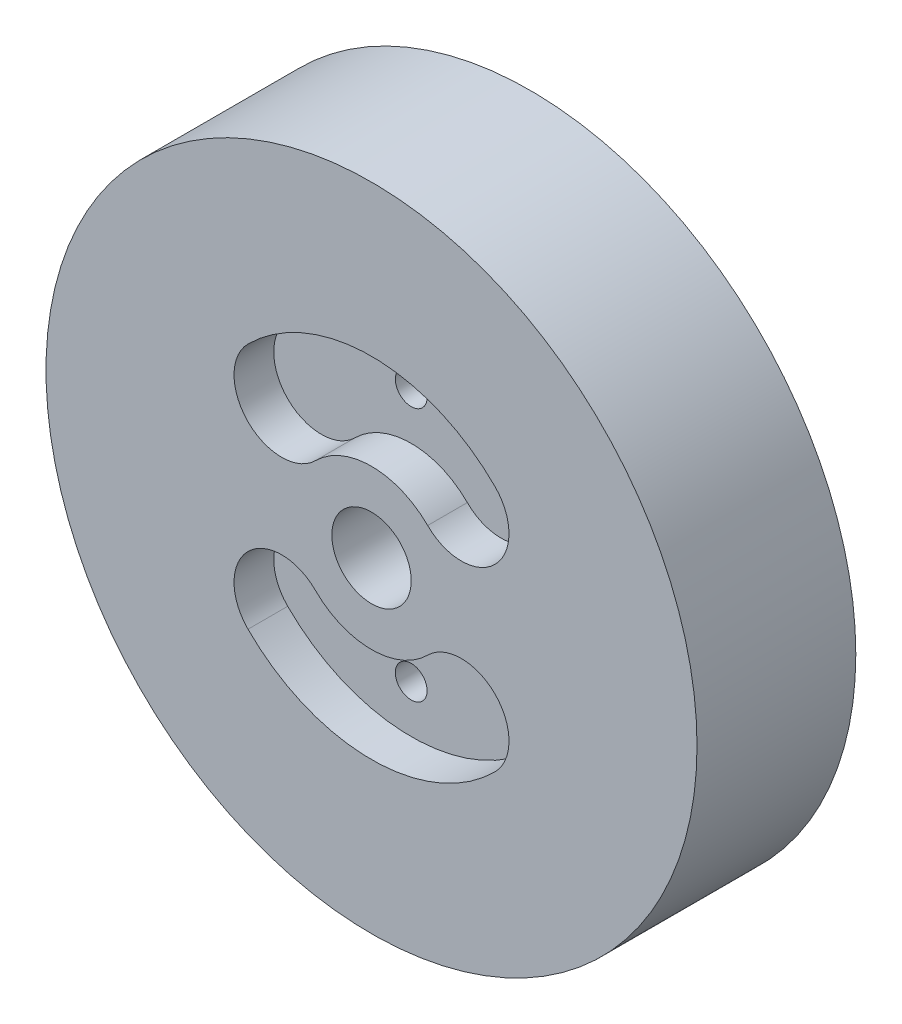
from build123d import *

# Parameters (mm, degrees)
DISC_PROFILE_41_R         = 20.5
PORT_BLOCK_DISC_DEPTH     = 10
ARC_PORT_SLOTS_DEPTH      = 2.5
THROUGH_PORTS_PROFILE_R   = 2.5
THROUGH_PORTS_PROFILE_R_2 = 1
THROUGH_PORTS_DEPTH       = 32.5
PORT_POCKETS_PROFILE_R    = 2.5
PORT_POCKETS_DEPTH        = 5


with BuildPart() as part:
    # Disc Profile Ø41 → Port Block Disc (new body)
    with BuildSketch(Plane.XY):
        Circle(DISC_PROFILE_41_R)
    extrude(amount=PORT_BLOCK_DISC_DEPTH)

    # Arc Port Slots Profile → Arc Port Slots (cut)
    with BuildSketch(Plane.XY.offset(10)):
        with BuildLine():
            ThreePointArc((7.778174593, 7.778174593), (0, 11), (-7.778174593, 7.778174593))
            ThreePointArc((-7.778174593, 7.778174593), (-7.778174593, 3.535533906), (-3.535533906, 3.535533906))
            ThreePointArc((-3.535533906, 3.535533906), (0, 5), (3.535533906, 3.535533906))
            ThreePointArc((3.535533906, 3.535533906), (7.778174593, 3.535533906), (7.778174593, 7.778174593))
        make_face()
        with BuildLine():
            ThreePointArc((3.535533906, -3.535533906), (0, -5), (-3.535533906, -3.535533906))
            ThreePointArc((-3.535533906, -3.535533906), (-7.778174593, -3.535533906), (-7.778174593, -7.778174593))
            ThreePointArc((-7.778174593, -7.778174593), (0, -11), (7.778174593, -7.778174593))
            ThreePointArc((7.778174593, -7.778174593), (7.778174593, -3.535533906), (3.535533906, -3.535533906))
        make_face()
    extrude(amount=-ARC_PORT_SLOTS_DEPTH, mode=Mode.SUBTRACT)

    # Through Ports Profile → Through Ports (cut)
    with BuildSketch(Plane.XY.offset(10)):
        Circle(THROUGH_PORTS_PROFILE_R)
        with Locations((0, 8)):
            Circle(THROUGH_PORTS_PROFILE_R_2)
        with Locations((0, -8)):
            Circle(THROUGH_PORTS_PROFILE_R_2)
    extrude(amount=-THROUGH_PORTS_DEPTH, mode=Mode.SUBTRACT)

    # Port Pockets Profile → Port Pockets (cut)
    with BuildSketch(Plane(origin=(0, 0, 0), x_dir=(-1, 0, 0), z_dir=(0, 0, -1))):
        with Locations((12.5, 0)):
            Circle(PORT_POCKETS_PROFILE_R)
        with Locations((-12.5, 0)):
            Circle(PORT_POCKETS_PROFILE_R)
    extrude(amount=-PORT_POCKETS_DEPTH, mode=Mode.SUBTRACT)


solid = part.part
